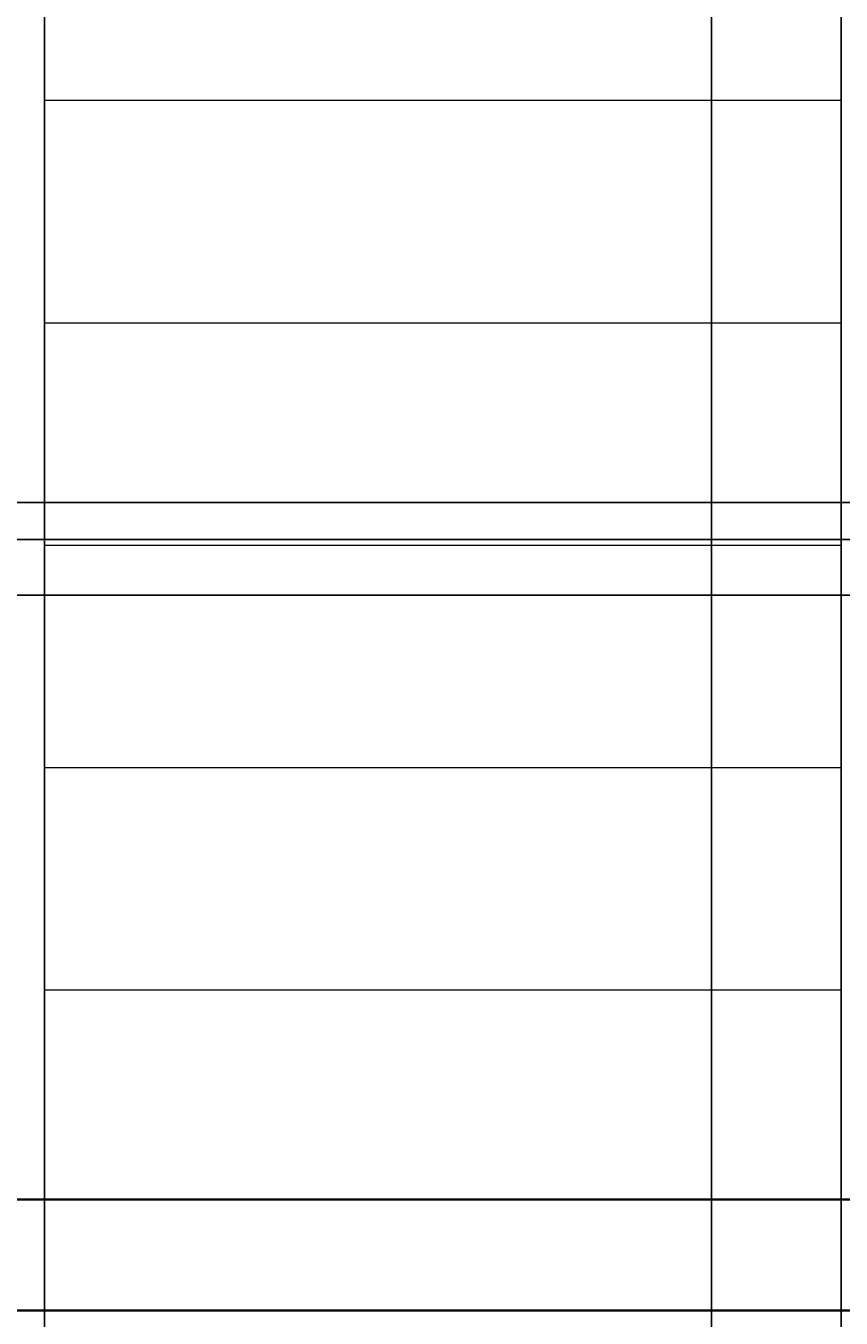
# Model space of a CAD drawing. Units: inches. Extents: x -6 to 289, y -8 to 323.
# Tile 68 of 107: x 212 to 234, y 159 to 194. Entities that reach past the tile are written whole.
import ezdxf

# ---------------------------------------------------------------- set-up
doc = ezdxf.new("R2010")
doc.units = ezdxf.units.IN
doc.header["$MEASUREMENT"] = 0
for name, color, linetype, lineweight in [('A-ANNO-DIMS', 2, 'Continuous', 18), ('A-ELEV', 7, 'Continuous', 35), ('A-ELEV-PATT', 8, 'Continuous', 13), ('A-GLAZ', 4, 'Continuous', 25)]:
    doc.layers.add(name, color=color, linetype=linetype, lineweight=lineweight)
doc.styles.get("Standard").update_dxf_attribs({"font": 'arial.ttf'})
doc.dimstyles.get("Standard").update_dxf_attribs({"dimtxt": 0.18, "dimasz": 0.18, "dimexe": 0.18, "dimexo": 0.0625, "dimgap": 0.09, "dimtad": 0, "dimtih": 1, "dimtoh": 1, "dimdec": 4, "dimzin": 0, "dimdsep": 46, "dimtxsty": 'Standard', "dimcen": 0.09, "dimadec": 0, "dimazin": 0, "dimtfac": 1, "dimtdec": 4, "dimtofl": 0, "dimtmove": 0, "dimatfit": 3, "dimfxl": 1, "dimtolj": 1, "dimtzin": 0, "dimarcsym": 0})

# ---------------------------------------------------------------- blocks, each defined once
blk = doc.blocks.new('*D24')
at = {"layer": 'A-ANNO-DIMS', "color": 0, "lineweight": -2, "transparency": 16777216}
for p, q in [((126.946, 178.654), (288.653, 178.654)), ((288.473, 178.474), (288.473, 159.153)), ((288.473, 139.469), (288.473, 158.789)), ((259.226, 139.289), (288.653, 139.289))]:
    blk.add_line(p, q, dxfattribs=at)
at = {"layer": 'A-ANNO-DIMS', "color": 0, "transparency": 16777216}
for points in [[(288.443, 178.474), (288.503, 178.474), (288.473, 178.654)], [(288.443, 139.469), (288.503, 139.469), (288.473, 139.289)]]:
    blk.add_solid(points, dxfattribs=at)
at = {"layer": 'Defpoints', "color": 0, "transparency": 16777216}
for p in [(126.883, 178.654), (288.473, 178.654), (259.164, 139.289)]:
    blk.add_point(p, dxfattribs=at)
at = {"layer": 'A-ANNO-DIMS', "color": 0, "transparency": 16777216, "insert": (288.473, 158.971), "char_height": 0.18, "attachment_point": 5}
blk.add_mtext('\\A1;39.365', dxfattribs=at)
blk = doc.blocks.new('*D25')
at = {"layer": 'A-ANNO-DIMS', "color": 0, "lineweight": -2, "transparency": 16777216}
for p, q in [((126.946, 226.654), (288.653, 226.654)), ((288.473, 226.474), (288.473, 202.836)), ((288.473, 178.834), (288.473, 202.472)), ((126.946, 178.654), (288.653, 178.654))]:
    blk.add_line(p, q, dxfattribs=at)
at = {"layer": 'A-ANNO-DIMS', "color": 0, "transparency": 16777216}
for points in [[(288.443, 226.474), (288.503, 226.474), (288.473, 226.654)], [(288.443, 178.834), (288.503, 178.834), (288.473, 178.654)]]:
    blk.add_solid(points, dxfattribs=at)
at = {"layer": 'Defpoints', "color": 0, "transparency": 16777216}
for p in [(126.883, 226.654), (288.473, 226.654), (126.883, 178.654)]:
    blk.add_point(p, dxfattribs=at)
at = {"layer": 'A-ANNO-DIMS', "color": 0, "transparency": 16777216, "insert": (288.473, 202.654), "char_height": 0.18, "attachment_point": 5}
blk.add_mtext('\\A1;48', dxfattribs=at)
blk = doc.blocks.new('*D35')
at = {"layer": 'A-ANNO-DIMS', "color": 0, "lineweight": -2, "transparency": 16777216}
for p, q in [((167.446, 180.154), (288.653, 180.154)), ((288.473, 179.974), (288.473, 179.586)), ((288.473, 178.834), (288.473, 179.222)), ((168.946, 178.654), (288.653, 178.654))]:
    blk.add_line(p, q, dxfattribs=at)
at = {"layer": 'A-ANNO-DIMS', "color": 0, "transparency": 16777216}
for points in [[(288.443, 179.974), (288.503, 179.974), (288.473, 180.154)], [(288.443, 178.834), (288.503, 178.834), (288.473, 178.654)]]:
    blk.add_solid(points, dxfattribs=at)
at = {"layer": 'Defpoints', "color": 0, "transparency": 16777216}
for p in [(167.383, 180.154), (288.473, 180.154), (168.883, 178.654)]:
    blk.add_point(p, dxfattribs=at)
at = {"layer": 'A-ANNO-DIMS', "color": 0, "transparency": 16777216, "insert": (288.473, 179.404), "char_height": 0.18, "attachment_point": 5}
blk.add_mtext('\\A1;1.5', dxfattribs=at)
blk = doc.blocks.new('*D36')
at = {"layer": 'A-ANNO-DIMS', "color": 0, "lineweight": -2, "transparency": 16777216}
for p, q in [((166.446, 181.154), (288.653, 181.154)), ((288.473, 180.974), (288.473, 180.834)), ((288.473, 180.334), (288.473, 180.474)), ((167.446, 180.154), (288.653, 180.154))]:
    blk.add_line(p, q, dxfattribs=at)
at = {"layer": 'A-ANNO-DIMS', "color": 0, "transparency": 16777216}
for points in [[(288.443, 180.974), (288.503, 180.974), (288.473, 181.154)], [(288.443, 180.334), (288.503, 180.334), (288.473, 180.154)]]:
    blk.add_solid(points, dxfattribs=at)
at = {"layer": 'Defpoints', "color": 0, "transparency": 16777216}
for p in [(166.383, 181.154), (288.473, 181.154), (167.383, 180.154)]:
    blk.add_point(p, dxfattribs=at)
at = {"layer": 'A-ANNO-DIMS', "color": 0, "transparency": 16777216, "insert": (288.473, 180.654), "char_height": 0.18, "attachment_point": 5}
blk.add_mtext('\\A1;1', dxfattribs=at)
blk = doc.blocks.new('*D37')
at = {"layer": 'A-ANNO-DIMS', "color": 0, "lineweight": -2, "transparency": 16777216}
for p, q in [((166.446, 224.154), (288.653, 224.154)), ((288.473, 223.974), (288.473, 202.836)), ((288.473, 181.334), (288.473, 202.472)), ((166.446, 181.154), (288.653, 181.154))]:
    blk.add_line(p, q, dxfattribs=at)
at = {"layer": 'A-ANNO-DIMS', "color": 0, "transparency": 16777216}
for points in [[(288.443, 223.974), (288.503, 223.974), (288.473, 224.154)], [(288.443, 181.334), (288.503, 181.334), (288.473, 181.154)]]:
    blk.add_solid(points, dxfattribs=at)
at = {"layer": 'Defpoints', "color": 0, "transparency": 16777216}
for p in [(166.383, 224.154), (288.473, 224.154), (166.383, 181.154)]:
    blk.add_point(p, dxfattribs=at)
at = {"layer": 'A-ANNO-DIMS', "color": 0, "transparency": 16777216, "insert": (288.473, 202.654), "char_height": 0.18, "attachment_point": 5}
blk.add_mtext('\\A1;43', dxfattribs=at)
blk = doc.blocks.new('*D43')
at = {"layer": 'A-ANNO-DIMS', "color": 0, "lineweight": -2, "transparency": 16777216}
for p, q in [((211.292, 224.326), (211.292, -8.391)), ((212.292, 224.326), (212.292, -8.391)), ((211.472, -8.211), (211.669, -8.211)), ((212.112, -8.211), (211.915, -8.211))]:
    blk.add_line(p, q, dxfattribs=at)
at = {"layer": 'A-ANNO-DIMS', "color": 0, "transparency": 16777216}
for points in [[(211.472, -8.181), (211.472, -8.241), (211.292, -8.211)], [(212.112, -8.181), (212.112, -8.241), (212.292, -8.211)]]:
    blk.add_solid(points, dxfattribs=at)
at = {"layer": 'Defpoints', "color": 0, "transparency": 16777216}
for p in [(211.292, 224.389), (212.292, 224.389), (212.292, -8.211)]:
    blk.add_point(p, dxfattribs=at)
at = {"layer": 'A-ANNO-DIMS', "color": 0, "transparency": 16777216, "insert": (211.792, -8.211), "char_height": 0.18, "attachment_point": 5}
blk.add_mtext('\\A1;1', dxfattribs=at)
blk = doc.blocks.new('*D44')
at = {"layer": 'A-ANNO-DIMS', "color": 0, "lineweight": -2, "transparency": 16777216}
for p, q in [((212.292, 224.326), (212.292, -8.391)), ((233.792, 224.326), (233.792, -8.391)), ((212.472, -8.211), (222.716, -8.211)), ((233.612, -8.211), (223.368, -8.211))]:
    blk.add_line(p, q, dxfattribs=at)
at = {"layer": 'A-ANNO-DIMS', "color": 0, "transparency": 16777216}
for points in [[(212.472, -8.181), (212.472, -8.241), (212.292, -8.211)], [(233.612, -8.181), (233.612, -8.241), (233.792, -8.211)]]:
    blk.add_solid(points, dxfattribs=at)
at = {"layer": 'Defpoints', "color": 0, "transparency": 16777216}
for p in [(212.292, 224.389), (233.792, 224.389), (233.792, -8.211)]:
    blk.add_point(p, dxfattribs=at)
at = {"layer": 'A-ANNO-DIMS', "color": 0, "transparency": 16777216, "insert": (223.042, -8.211), "char_height": 0.18, "attachment_point": 5}
blk.add_mtext('\\A1;21.5', dxfattribs=at)
blk = doc.blocks.new('*D80')
at = {"layer": 'A-ANNO-DIMS', "color": 0, "lineweight": -2, "transparency": 16777216}
for p, q in [((188.292, 116.842), (188.292, 322.969)), ((230.292, 116.842), (230.292, 322.969)), ((188.472, 322.789), (209.07, 322.789)), ((230.112, 322.789), (209.513, 322.789))]:
    blk.add_line(p, q, dxfattribs=at)
at = {"layer": 'A-ANNO-DIMS', "color": 0, "transparency": 16777216}
for points in [[(188.472, 322.819), (188.472, 322.759), (188.292, 322.789)], [(230.112, 322.819), (230.112, 322.759), (230.292, 322.789)]]:
    blk.add_solid(points, dxfattribs=at)
at = {"layer": 'Defpoints', "color": 0, "transparency": 16777216}
for p in [(230.292, 322.789), (188.292, 116.779), (230.292, 116.779)]:
    blk.add_point(p, dxfattribs=at)
at = {"layer": 'A-ANNO-DIMS', "color": 0, "transparency": 16777216, "insert": (209.292, 322.789), "char_height": 0.18, "attachment_point": 5}
blk.add_mtext('\\A1;42', dxfattribs=at)
blk = doc.blocks.new('*D81')
at = {"layer": 'A-ANNO-DIMS', "color": 0, "lineweight": -2, "transparency": 16777216}
for p, q in [((230.292, 68.842), (230.292, 322.969)), ((245.215, 66.286), (245.215, 322.969)), ((230.472, 322.789), (237.298, 322.789)), ((245.035, 322.789), (238.208, 322.789))]:
    blk.add_line(p, q, dxfattribs=at)
at = {"layer": 'A-ANNO-DIMS', "color": 0, "transparency": 16777216}
for points in [[(230.472, 322.819), (230.472, 322.759), (230.292, 322.789)], [(245.035, 322.819), (245.035, 322.759), (245.215, 322.789)]]:
    blk.add_solid(points, dxfattribs=at)
at = {"layer": 'Defpoints', "color": 0, "transparency": 16777216}
for p in [(245.215, 322.789), (230.292, 68.779), (245.215, 66.224)]:
    blk.add_point(p, dxfattribs=at)
at = {"layer": 'A-ANNO-DIMS', "color": 0, "transparency": 16777216, "insert": (237.753, 322.789), "char_height": 0.18, "attachment_point": 5}
blk.add_mtext('\\A1;14.923', dxfattribs=at)
blk = doc.blocks.new('*D98')
at = {"layer": 'A-ANNO-DIMS', "color": 0, "lineweight": -2, "transparency": 16777216}
for p, q in [((202.741, 159.411), (202.741, 322.969)), ((244.164, 159.411), (244.164, 322.969)), ((202.921, 322.789), (223.056, 322.789)), ((243.984, 322.789), (223.849, 322.789))]:
    blk.add_line(p, q, dxfattribs=at)
at = {"layer": 'A-ANNO-DIMS', "color": 0, "transparency": 16777216}
for points in [[(202.921, 322.819), (202.921, 322.759), (202.741, 322.789)], [(243.984, 322.819), (243.984, 322.759), (244.164, 322.789)]]:
    blk.add_solid(points, dxfattribs=at)
at = {"layer": 'Defpoints', "color": 0, "transparency": 16777216}
for p in [(244.164, 322.789), (202.741, 159.348), (244.164, 159.348)]:
    blk.add_point(p, dxfattribs=at)
at = {"layer": 'A-ANNO-DIMS', "color": 0, "transparency": 16777216, "insert": (223.452, 322.789), "char_height": 0.18, "attachment_point": 5}
blk.add_mtext('\\A1;41.42', dxfattribs=at)

msp = doc.modelspace()

# ---------------------------------------------------------------- hatches: boundary and pattern name
at = {"layer": 'A-ELEV-PATT'}
h = msp.add_hatch(dxfattribs=at)
h.set_pattern_fill('_USER', color=256, scale=6, pattern_type=0)
h.set_pattern_definition([(0, (0, 0), (0, 6), [])])
h.paths.add_polyline_path([(184.1244, 48.0851), (124.008, 48.0851), (124.008, 10.2888), (184.1244, 10.2888)])
h.paths.add_polyline_path([(244.2408, 48.0851), (186.3604, 48.0851), (186.3604, 10.2888), (244.2408, 10.2888)])
h.paths.add_polyline_path([(208.2918, 114.2795), (190.7918, 114.2795), (190.7918, 71.2795), (208.2918, 71.2795)])
h.paths.add_polyline_path([(227.7918, 114.2795), (209.2918, 114.2795), (209.2918, 71.2795), (227.7918, 71.2795)])
h.paths.add_polyline_path([(211.2918, 224.3887), (190.7918, 224.3887), (190.7918, 162.3484), (211.2918, 162.3484)])
h.paths.add_polyline_path([(233.7918, 224.3887), (212.2918, 224.3887), (212.2918, 162.3484), (233.7918, 162.3484)])
h.paths.add_polyline_path([(166.3835, 224.154), (147.8835, 224.154), (147.8835, 181.154), (166.3835, 181.154)])
h.paths.add_polyline_path([(146.8835, 224.154), (129.3835, 224.154), (129.3835, 181.154), (146.8835, 181.154)])

# ---------------------------------------------------------------- linework, layer by layer
at = {"layer": 'A-ELEV'}
for points in [[(247.1638, 139.2888), (115.1638, 139.2888), (115.1638, 162.3484), (247.1638, 162.3484)], [(244.1638, 142.2888), (118.1638, 142.2888), (118.1638, 159.3484), (244.1638, 159.3484)]]:
    msp.add_lwpolyline(points, close=True, dxfattribs=at)
at = {"layer": 'A-GLAZ'}
msp.add_line((212.2918, 162.3484), (212.2918, 225.3887), dxfattribs=at)
msp.add_lwpolyline([(212.2918, 224.3887), (233.7918, 224.3887), (233.7918, 162.3484)], dxfattribs=at)

# ---------------------------------------------------------------- dimensions: what is measured, and where the dimension line sits
at = {"layer": 'A-ANNO-DIMS'}
for base, p1, p2, override, picture, middle in [((230.2918, 322.7888), (188.2918, 116.7795), (230.2918, 116.7795), {"dimdec": 0, "dimlfac": 1, "dimrnd": 0, "dimzin": 0, "dimdsep": 46, "dimlunit": 2}, '*D80', (209.2918, 322.7888)), ((244.1638, 322.7888), (202.741, 159.3484), (244.1638, 159.3484), {"dimdec": 2, "dimlfac": 1, "dimrnd": 0, "dimzin": 0, "dimdsep": 46, "dimlunit": 2}, '*D98', (223.4524, 322.7888)), ((245.2146, 322.7888), (230.2918, 68.7795), (245.2146, 66.2238), {"dimdec": 3, "dimlfac": 1, "dimrnd": 0, "dimzin": 0, "dimdsep": 46, "dimlunit": 2}, '*D81', (237.7532, 322.7888)), ((212.2918, -8.2112), (211.2918, 224.3887), (212.2918, 224.3887), {"dimdec": 0, "dimlfac": 1, "dimrnd": 0, "dimzin": 0, "dimdsep": 46, "dimlunit": 2}, '*D43', (211.7918, -8.2112)), ((233.7918, -8.2112), (212.2918, 224.3887), (233.7918, 224.3887), {"dimdec": 1, "dimlfac": 1, "dimrnd": 0, "dimzin": 0, "dimdsep": 46, "dimlunit": 2}, '*D44', (223.0418, -8.2112))]:
    dim = msp.add_linear_dim(base=base, p1=p1, p2=p2, dimstyle='Standard', override=override, dxfattribs=at)
    dim.commit()
    dim.dimension.update_dxf_attribs({"geometry": picture, "text_midpoint": middle})
for base, p1, p2, override, picture, middle in [((288.4733, 226.654), (126.8835, 178.654), (126.8835, 226.654), {"dimdec": 0, "dimlfac": 1, "dimrnd": 0, "dimzin": 0, "dimdsep": 46, "dimlunit": 2}, '*D25', (288.4733, 202.654)), ((288.4733, 224.154), (166.3835, 181.154), (166.3835, 224.154), {"dimdec": 0, "dimlfac": 1, "dimrnd": 0, "dimzin": 0, "dimdsep": 46, "dimlunit": 2}, '*D37', (288.4733, 202.654)), ((288.4733, 181.154), (167.3835, 180.154), (166.3835, 181.154), {"dimdec": 0, "dimlfac": 1, "dimrnd": 0, "dimzin": 0, "dimdsep": 46, "dimlunit": 2}, '*D36', (288.4733, 180.654)), ((288.4733, 180.154), (168.8835, 178.654), (167.3835, 180.154), {"dimdec": 1, "dimlfac": 1, "dimrnd": 0, "dimzin": 0, "dimdsep": 46, "dimlunit": 2}, '*D35', (288.4733, 179.404)), ((288.4733, 178.654), (259.1638, 139.2888), (126.8835, 178.654), {"dimdec": 3, "dimlfac": 1, "dimrnd": 0, "dimzin": 0, "dimdsep": 46, "dimlunit": 2}, '*D24', (288.4733, 158.9714))]:
    dim = msp.add_linear_dim(base=base, p1=p1, p2=p2, angle=90, dimstyle='Standard', override=override, dxfattribs=at)
    dim.commit()
    dim.dimension.update_dxf_attribs({"geometry": picture, "text_midpoint": middle})

doc.saveas('drawing.dxf')
